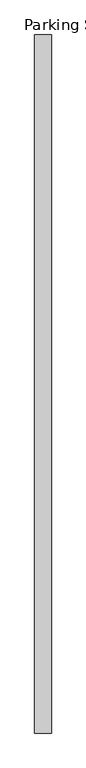
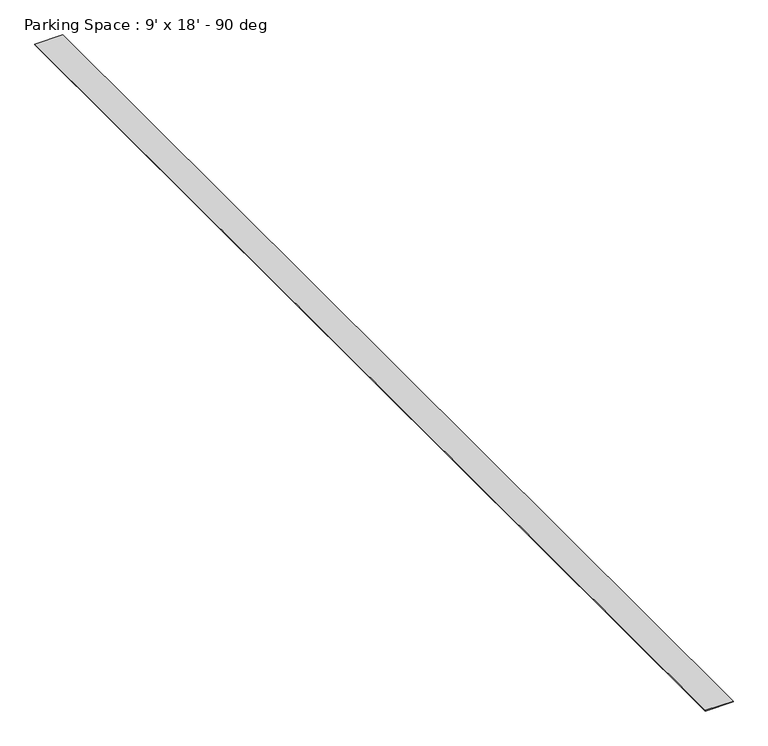
"""IFC4 building model written with IfcOpenShell, lengths in millimetres: proxy geometry, Parking Space : 9' x 18' - 90 deg."""

from ifc_helpers import new_model, si_unit, origin, origin_with_axes, place, context, project, spatial, polyline, outline, extrude, source, transform, mapped, element, save


def parking_space_9_x_18_90_deg_fdd9e8f5(model_context):
    return source(origin(), model_context, "Body", "SweptSolid", [
        extrude(outline(polyline([(-50.8, 0.0), (50.8, 0.0), (50.8, -4267.2), (-50.8, -4267.2), (-50.8, 0.0)])), origin_with_axes(), (0.0, 0.0, 1.0), 3.175),
    ])


if __name__ == "__main__":
    model = new_model("IFC4")
    model_context = context("Model", 3, world=origin())
    ifc_project = project(units=[si_unit("LENGTHUNIT", "METRE", prefix="MILLI")], contexts=[model_context])
    site = spatial("IfcSite", under=ifc_project)
    building = spatial("IfcBuilding", under=site)
    placement = place(None, origin())
    parking_space_9_x_18_90_deg_shape = parking_space_9_x_18_90_deg_fdd9e8f5(model_context)
    element("IfcBuildingElementProxy", 1, Name="Parking Space : 9' x 18' - 90 deg", ObjectType="Parking Space : 9' x 18' - 90 deg", at=placement, inside=building, context=model_context, shape_type="MappedRepresentation", body=[
        mapped(parking_space_9_x_18_90_deg_shape, transform((0.0, 0.0, 0.0), x_axis=(1.0, 0.0, 0.0), y_axis=(0.0, 1.0, 0.0), z_axis=(0.0, 0.0, 1.0))),
    ])
    save(model, "model.ifc")

# Revit data of these elements
# Type "Parking Space : 9' x 18' - 90 deg"
#   Angle = 90.00°
#   Parking Length = 18' - 0"
#   Parking Width = 9' - 0"
#   pl = 14' - 0"
#   pw = 7' - 0"
# Element 1 (IfcBuildingElementProxy, "Parking Space : 9' x 18' - 90 deg")
#   Materials on its faces: "Parking Stripe"
# Materials
#   "Parking Stripe": class "Paint", colour RGB 250 250 91, transparency 0
